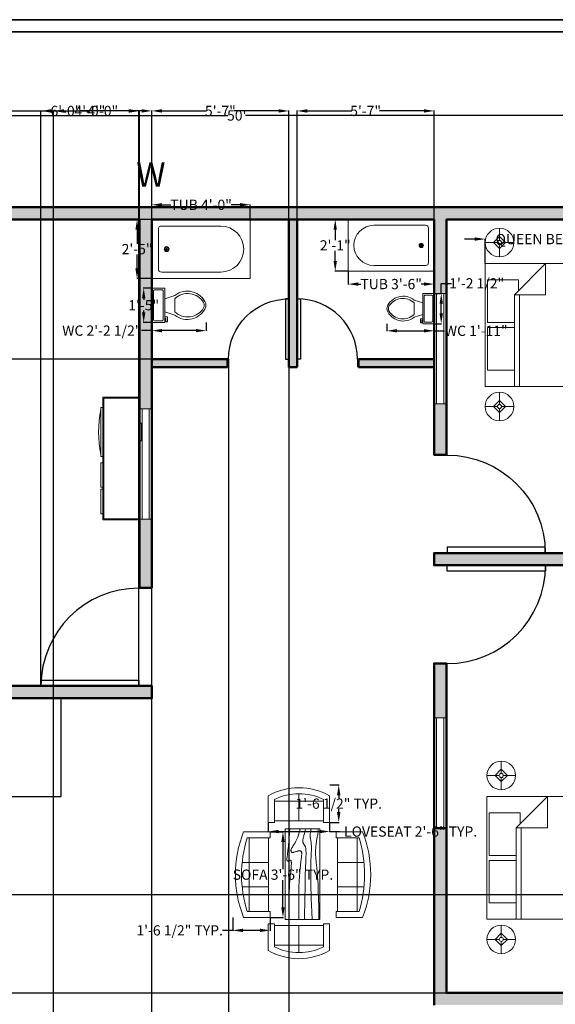
# Model space of a CAD drawing. Units: inches. Extents: x -60 to 743, y -483 to 510.
# Tile 6 of 7: x 209 to 470, y 29 to 510. Entities that reach past the tile are written whole.
import ezdxf

# ---------------------------------------------------------------- set-up
doc = ezdxf.new("R2010")
doc.units = ezdxf.units.IN
doc.header["$MEASUREMENT"] = 0
for name, color, linetype, lineweight in [('A-ANNO-DIMS', 2, 'Continuous', 18), ('A-ANNO-SYMB', 7, 'Continuous', 18), ('A-ANNO-TTLB', 7, 'Continuous', 35), ('A-DOOR', 150, 'Continuous', 25), ('A-FLOR-FIXT', 40, 'Continuous', 18), ('A-WALL-PATT', 30, 'Continuous', 13), ('FURNITURE', 40, 'Continuous', 18), ('STAIRS', 202, 'Continuous', 25), ('WALL BOUNDRY', 10, 'Continuous', 50), ('WINDOW', 200, 'Continuous', 18)]:
    doc.layers.add(name, color=color, linetype=linetype, lineweight=lineweight)
doc.styles.get("Standard").update_dxf_attribs({"font": 'arial.ttf'})
doc.dimstyles.get("Standard").update_dxf_attribs({"dimtxt": 5, "dimasz": 5, "dimexe": 0.18, "dimexo": 0.0625, "dimgap": 0.09, "dimtad": 0, "dimtih": 1, "dimtoh": 1, "dimdec": 1, "dimzin": 0, "dimdsep": 46, "dimlunit": 4, "dimtxsty": 'Standard', "dimcen": 0.09, "dimadec": 0, "dimazin": 0, "dimtfac": 1, "dimtdec": 1, "dimtofl": 0, "dimtmove": 0, "dimatfit": 3, "dimfxl": 1, "dimtolj": 1, "dimtzin": 0, "dimarcsym": 0})

# ---------------------------------------------------------------- blocks, each defined once
blk = doc.blocks.new('*U5')
for p, q in [((0, 0), (0, -100)), ((750, 0), (750, -100))]:
    blk.add_line(p, q)
blk.add_lwpolyline([(0, 0), (0, 750), (43.75, 750), (43.75, 0)], close=True)
blk.add_arc((0, 0), 750, 0, 90)
blk = doc.blocks.new('Sofa - Roundback 7 ft.')
for p, q in [((-12.00002, -32.4421), (-12.00003, -6.5971)), ((11.99997, -32.4421), (11.99998, -6.5971)), ((-36.000027, -34), (-36.000027, -11.4696)), ((-35.999844, -13.3819), (35.9998, -13.3819)), ((35.99998, -34), (35.99998, -11.4696)), ((-36.000027, -32.4421), (35.99998, -32.4421))]:
    blk.add_line(p, q)
for points in [[(-36.000027, -34), (-42.000027, -34), (-42.000027, -8)], [(41.99998, -8), (41.99998, -34), (35.99998, -34)]]:
    blk.add_lwpolyline(points)
for centre, radius, start, end in [((0, -114.25), 114.25, 68.43141, 111.5686), ((-0.00001, -127.1968), 121.1968, 72.72033, 107.2797)]:
    blk.add_arc(centre, radius, start, end)
blk = doc.blocks.new('Sofa - Roundback Loveseat 5 ft.')
for p, q in [((0, -32.44198), (0, -5.99998)), ((-24, -33.99998), (-24, -11.46958)), ((-23.9998, -13.38178), (23.99986, -13.38178)), ((24.00004, -33.99998), (24.00004, -11.46958)), ((-24, -32.44198), (24.00004, -32.44198))]:
    blk.add_line(p, q)
for points in [[(-24, -33.99998), (-30, -33.99998), (-30, -7.99998)], [(30.00004, -7.99998), (30.00004, -33.99998), (24.00004, -33.99998)]]:
    blk.add_lwpolyline(points)
for centre, radius, start, end in [((0, -60.24998), 60.24998, 60.13715, 119.8628), ((0, -61.38438), 55.38444, 64.32083, 115.6792)]:
    blk.add_arc(centre, radius, start, end)
blk = doc.blocks.new('Lamp - Table')
for p, q in [((0, 7), (0, 1)), ((-1, 0), (-7, 0)), ((0, 3), (-3, 0)), ((-3, 0), (0, -3)), ((3, 0), (0, 3)), ((0, -3), (3, 0)), ((1, 0), (7, 0)), ((0, -1), (0, -7))]:
    blk.add_line(p, q)
for radius in [7, 1]:
    blk.add_circle((0, 0), radius)
blk = doc.blocks.new('Bed - Queen')
for p, q in [((0, -80.00003), (0, 0)), ((0, 0), (59.99999, 0)), ((59.99999, 0), (59.99999, -80.00003)), ((7.99999, -1.2), (28.79998, -1.2)), ((7.99999, -14.4), (7.99999, -1.2)), ((28.79998, -1.2), (28.79998, -14.4)), ((31.19999, -1.2), (51.99999, -1.2)), ((31.19999, -14.4), (31.19999, -1.2)), ((51.99999, -1.2), (51.99999, -16.4)), ((0, -14.4), (44.8, -14.4)), ((59.99999, -29.6), (44.8, -14.4)), ((44.8, -14.4), (44.8, -29.6)), ((44.8, -16.8), (0, -16.8)), ((51.99999, -16.4), (46.79936, -16.4)), ((44.8, -29.6), (59.99999, -29.6)), ((59.99999, -80.00003), (0, -80.00003))]:
    blk.add_line(p, q)
blk = doc.blocks.new('Bath Tub - 26 x 60 in.')
for p, q in [((9, -17), (9, -19)), ((8, -18), (10, -18))]:
    blk.add_line(p, q)
blk.add_lwpolyline([(0, -36), (0, 0), (60, 0), (60, -36)], close=True)
for points in [[(6, -4), (42, -4)], [(4, -30), (4, -6)], [(42, -32), (6, -32)]]:
    blk.add_lwpolyline(points)
for radius in [1.5, 1]:
    blk.add_circle((9, -18), radius)
for centre, radius, start, end in [((5.75, -5.75), 1.77, 81.8699, 188.1301), ((42, -18), 14, 270, 90), ((5.75, -30.25), 1.77, 171.8699, 278.1301)]:
    blk.add_arc(centre, radius, start, end)
blk = doc.blocks.new('Toilet - top')
for p, q in [((9.5, -6), (9.5, -2)), ((-10, -8.5), (-8, -8.5)), ((-10, -9.5), (-10, -8.5)), ((-7, -9.5), (-10, -9.5)), ((-8, -8.5), (-8, -8)), ((-7, -8), (-7, -9.5)), ((-4, -8), (-6, -14)), ((4, -8), (6, -14)), ((4, -14), (-4, -14))]:
    blk.add_line(p, q)
blk.add_lwpolyline([(10.5, -8), (10.5, 0), (-10.5, 0), (-10.5, -8)], close=True)
for points in [[(-9.5, -2), (-9.5, -6)], [(8.5, -1), (-8.5, -1)], [(-8.5, -7), (8.5, -7)]]:
    blk.add_lwpolyline(points)
for centre, radius, start, end in [((-8.62, -1.88), 0.884, 81.8699, 188.1301), ((8.62, -1.88), 0.884, 351.8699, 98.1301), ((-8.62, -6.12), 0.884, 171.8699, 278.1301), ((8.62, -6.12), 0.884, 261.8699, 8.1301), ((3.52, -21.58), 12.17, 141.46911, 247.97143), ((4.2, -21.82), 11.33, 136.36773, 238.94682), ((-3.52, -21.58), 12.17, 292.02843, 38.53071), ((-4.2, -21.82), 11.33, 301.05301, 43.63209), ((0, -27.88), 4, 245.73182, 294.26817), ((0, -29), 4, 254.86053, 285.13947)]:
    blk.add_arc(centre, radius, start, end)
blk = doc.blocks.new('Entertainment Center')
for p, q in [((-4, 0), (-5, -1)), ((4, 0), (-4, 0)), ((5, -1), (4, 0)), ((-17, -19), (-17, -1)), ((-17, -1), (43, -1)), ((-16.5, -18.5), (-16.5, -1.5)), ((-16.5, -1.5), (42.5, -1.5)), ((42.5, -1.5), (42.5, -18.5)), ((43, -1), (43, -19)), ((43, -19), (-17, -19)), ((42.5, -18.5), (-16.5, -18.5)), ((-12, -20), (-12, -19)), ((12, -19), (12, -20)), ((15, -20), (15, -19)), ((27, -19), (27, -20)), ((28, -20), (28, -19)), ((40, -19), (40, -20)), ((12, -20), (-12, -20)), ((27, -20), (15, -20)), ((40, -20), (28, -20))]:
    blk.add_line(p, q)
blk.add_arc((0, 40), 61, 259.6111, 280.3889)
blk = doc.blocks.new('*D22')
at = {"layer": 'A-ANNO-DIMS', "color": 0, "lineweight": -2, "transparency": 16777216}
for p, q in [((13.15, 418.48), (13.15, 463.48)), ((18.15, 463.3), (310.31, 463.3)), ((611.15, 463.3), (318.98, 463.3)), ((616.15, 418.48), (616.15, 463.48))]:
    blk.add_line(p, q, dxfattribs=at)
at = {"layer": 'A-ANNO-DIMS', "color": 0, "transparency": 16777216}
for points in [[(18.15, 464.13), (18.15, 462.46), (13.15, 463.3)], [(611.15, 464.13), (611.15, 462.46), (616.15, 463.3)]]:
    blk.add_solid(points, dxfattribs=at)
at = {"layer": 'Defpoints', "color": 0, "transparency": 16777216}
for p in [(616.15, 463.3), (13.15, 418.42), (616.15, 418.42)]:
    blk.add_point(p, dxfattribs=at)
at = {"layer": 'A-ANNO-DIMS', "color": 0, "transparency": 16777216, "insert": (314.65, 463.3), "char_height": 5, "attachment_point": 5}
blk.add_mtext("\\A1;50'", dxfattribs=at)
blk = doc.blocks.new('*D40')
at = {"layer": 'A-ANNO-DIMS', "color": 0, "lineweight": -2, "transparency": 16777216}
for p, q in [((273.15, 412.48), (273.15, 419.82)), ((278.15, 419.64), (282.46, 419.64)), ((316.28, 419.64), (311.97, 419.64)), ((321.28, 412.48), (321.28, 419.82))]:
    blk.add_line(p, q, dxfattribs=at)
at = {"layer": 'A-ANNO-DIMS', "color": 0, "transparency": 16777216}
for points in [[(278.15, 420.48), (278.15, 418.81), (273.15, 419.64)], [(316.28, 420.48), (316.28, 418.81), (321.28, 419.64)]]:
    blk.add_solid(points, dxfattribs=at)
at = {"layer": 'Defpoints', "color": 0, "transparency": 16777216}
for p in [(321.28, 419.64), (273.15, 412.42), (321.28, 412.42)]:
    blk.add_point(p, dxfattribs=at)
at = {"layer": 'A-ANNO-DIMS', "color": 0, "transparency": 16777216, "insert": (297.21, 419.64), "char_height": 5, "attachment_point": 5}
blk.add_mtext('\\A1;TUB 4\'-0"', dxfattribs=at)
blk = doc.blocks.new('*D41')
at = {"layer": 'A-ANNO-DIMS', "color": 0, "lineweight": -2, "transparency": 16777216}
for p, q in [((273.08, 412.42), (265.75, 412.42)), ((265.93, 407.42), (265.93, 400.62)), ((265.93, 388.54), (265.93, 395.34)), ((273.08, 383.54), (265.75, 383.54))]:
    blk.add_line(p, q, dxfattribs=at)
at = {"layer": 'A-ANNO-DIMS', "color": 0, "transparency": 16777216}
for points in [[(265.09, 407.42), (266.76, 407.42), (265.93, 412.42)], [(265.09, 388.54), (266.76, 388.54), (265.93, 383.54)]]:
    blk.add_solid(points, dxfattribs=at)
at = {"layer": 'Defpoints', "color": 0, "transparency": 16777216}
for p in [(265.93, 412.42), (273.15, 412.42), (273.15, 383.54)]:
    blk.add_point(p, dxfattribs=at)
at = {"layer": 'A-ANNO-DIMS', "color": 0, "transparency": 16777216, "insert": (265.93, 397.98), "char_height": 5, "attachment_point": 5}
blk.add_mtext('\\A1;2\'-5"', dxfattribs=at)
blk = doc.blocks.new('*D42')
at = {"layer": 'A-ANNO-DIMS', "color": 0, "lineweight": -2, "transparency": 16777216}
for p, q in [((369.11, 387.13), (369.11, 380.71)), ((411.15, 387.13), (411.15, 380.71)), ((374.11, 380.89), (375.37, 380.89)), ((406.15, 380.89), (404.88, 380.89))]:
    blk.add_line(p, q, dxfattribs=at)
at = {"layer": 'A-ANNO-DIMS', "color": 0, "transparency": 16777216}
for points in [[(374.11, 381.72), (374.11, 380.06), (369.11, 380.89)], [(406.15, 381.72), (406.15, 380.06), (411.15, 380.89)]]:
    blk.add_solid(points, dxfattribs=at)
at = {"layer": 'Defpoints', "color": 0, "transparency": 16777216}
for p in [(369.11, 387.2), (411.15, 387.2), (369.11, 380.89)]:
    blk.add_point(p, dxfattribs=at)
at = {"layer": 'A-ANNO-DIMS', "color": 0, "transparency": 16777216, "insert": (390.13, 380.89), "char_height": 5, "attachment_point": 5}
blk.add_mtext('\\A1;TUB 3\'-6"', dxfattribs=at)
blk = doc.blocks.new('*D43')
at = {"layer": 'A-ANNO-DIMS', "color": 0, "lineweight": -2, "transparency": 16777216}
for p, q in [((369.04, 412.42), (362.62, 412.42)), ((362.8, 407.42), (362.8, 402.41)), ((362.8, 392.2), (362.8, 397.21)), ((369.04, 387.2), (362.62, 387.2))]:
    blk.add_line(p, q, dxfattribs=at)
at = {"layer": 'A-ANNO-DIMS', "color": 0, "transparency": 16777216}
for points in [[(361.97, 407.42), (363.63, 407.42), (362.8, 412.42)], [(361.97, 392.2), (363.63, 392.2), (362.8, 387.2)]]:
    blk.add_solid(points, dxfattribs=at)
at = {"layer": 'Defpoints', "color": 0, "transparency": 16777216}
for p in [(362.8, 412.42), (369.11, 412.42), (369.11, 387.2)]:
    blk.add_point(p, dxfattribs=at)
at = {"layer": 'A-ANNO-DIMS', "color": 0, "transparency": 16777216, "insert": (362.8, 399.81), "char_height": 5, "attachment_point": 5}
blk.add_mtext('\\A1;2\'-1"', dxfattribs=at)
blk = doc.blocks.new('*D46')
at = {"layer": 'A-ANNO-DIMS', "color": 0, "lineweight": -2, "transparency": 16777216}
for p, q in [((273.15, 362.04), (273.15, 357.95)), ((299.66, 362.04), (299.66, 357.95)), ((273.15, 358.13), (268.15, 358.13)), ((294.66, 358.13), (278.15, 358.13))]:
    blk.add_line(p, q, dxfattribs=at)
at = {"layer": 'A-ANNO-DIMS', "color": 0, "transparency": 16777216}
for points in [[(278.15, 358.96), (278.15, 357.3), (273.15, 358.13)], [(294.66, 358.96), (294.66, 357.3), (299.66, 358.13)]]:
    blk.add_solid(points, dxfattribs=at)
at = {"layer": 'Defpoints', "color": 0, "transparency": 16777216}
for p in [(273.15, 362.11), (299.66, 362.11), (273.15, 358.13)]:
    blk.add_point(p, dxfattribs=at)
at = {"layer": 'A-ANNO-DIMS', "color": 0, "transparency": 16777216, "insert": (248.69, 358.13), "char_height": 5, "attachment_point": 5}
blk.add_mtext('\\A1;WC 2\'-2 1/2"', dxfattribs=at)
blk = doc.blocks.new('*D47')
at = {"layer": 'A-ANNO-DIMS', "color": 0, "lineweight": -2, "transparency": 16777216}
for p, q in [((273.08, 378.95), (268.99, 378.95)), ((269.17, 373.95), (269.17, 373.17)), ((269.17, 367.11), (269.17, 367.89)), ((273.08, 362.11), (268.99, 362.11))]:
    blk.add_line(p, q, dxfattribs=at)
at = {"layer": 'A-ANNO-DIMS', "color": 0, "transparency": 16777216}
for points in [[(268.34, 373.95), (270, 373.95), (269.17, 378.95)], [(268.34, 367.11), (270, 367.11), (269.17, 362.11)]]:
    blk.add_solid(points, dxfattribs=at)
at = {"layer": 'Defpoints', "color": 0, "transparency": 16777216}
for p in [(269.17, 378.95), (273.15, 378.95), (273.15, 362.11)]:
    blk.add_point(p, dxfattribs=at)
at = {"layer": 'A-ANNO-DIMS', "color": 0, "transparency": 16777216, "insert": (269.17, 370.53), "char_height": 5, "attachment_point": 5}
blk.add_mtext('\\A1;1\'-5"', dxfattribs=at)
blk = doc.blocks.new('*D48')
at = {"layer": 'A-ANNO-DIMS', "color": 0, "lineweight": -2, "transparency": 16777216}
for p, q in [((387.99, 361.46), (387.99, 357.87)), ((411.15, 361.46), (411.15, 357.87)), ((392.99, 358.05), (406.15, 358.05)), ((411.15, 358.05), (416.15, 358.05))]:
    blk.add_line(p, q, dxfattribs=at)
at = {"layer": 'A-ANNO-DIMS', "color": 0, "transparency": 16777216}
for points in [[(392.99, 358.88), (392.99, 357.22), (387.99, 358.05)], [(406.15, 358.88), (406.15, 357.22), (411.15, 358.05)]]:
    blk.add_solid(points, dxfattribs=at)
at = {"layer": 'Defpoints', "color": 0, "transparency": 16777216}
for p in [(387.99, 361.52), (411.15, 361.52), (411.15, 358.05)]:
    blk.add_point(p, dxfattribs=at)
at = {"layer": 'A-ANNO-DIMS', "color": 0, "transparency": 16777216, "insert": (431.72, 358.05), "char_height": 5, "attachment_point": 5}
blk.add_mtext('\\A1;WC 1\'-11"', dxfattribs=at)
blk = doc.blocks.new('*D49')
at = {"layer": 'A-ANNO-DIMS', "color": 0, "lineweight": -2, "transparency": 16777216}
for p, q in [((414.62, 376.24), (414.62, 381.24)), ((414.62, 381.24), (419.62, 381.24)), ((411.21, 376.24), (414.8, 376.24)), ((414.62, 366.52), (414.62, 371.24)), ((411.21, 361.52), (414.8, 361.52))]:
    blk.add_line(p, q, dxfattribs=at)
at = {"layer": 'A-ANNO-DIMS', "color": 0, "transparency": 16777216}
for points in [[(413.79, 371.24), (415.45, 371.24), (414.62, 376.24)], [(413.79, 366.52), (415.45, 366.52), (414.62, 361.52)]]:
    blk.add_solid(points, dxfattribs=at)
at = {"layer": 'Defpoints', "color": 0, "transparency": 16777216}
for p in [(411.15, 376.24), (414.62, 376.24), (411.15, 361.52)]:
    blk.add_point(p, dxfattribs=at)
at = {"layer": 'A-ANNO-DIMS', "color": 0, "transparency": 16777216, "insert": (431.95, 381.24), "char_height": 5, "attachment_point": 5}
blk.add_mtext('\\A1;1\'-2 1/2"', dxfattribs=at)
blk = doc.blocks.new('*D50')
at = {"layer": 'A-ANNO-DIMS', "color": 0, "lineweight": -2, "transparency": 16777216}
for p, q in [((431.03, 402.88), (426.03, 402.88)), ((436.03, 390.95), (436.03, 403.06)), ((516.03, 390.95), (516.03, 403.06)), ((521.03, 402.88), (526.03, 402.88))]:
    blk.add_line(p, q, dxfattribs=at)
at = {"layer": 'A-ANNO-DIMS', "color": 0, "transparency": 16777216}
for points in [[(431.03, 403.72), (431.03, 402.05), (436.03, 402.88)], [(521.03, 403.72), (521.03, 402.05), (516.03, 402.88)]]:
    blk.add_solid(points, dxfattribs=at)
at = {"layer": 'Defpoints', "color": 0, "transparency": 16777216}
for p in [(436.03, 402.88), (436.03, 390.88), (516.03, 390.88)]:
    blk.add_point(p, dxfattribs=at)
at = {"layer": 'A-ANNO-DIMS', "color": 0, "transparency": 16777216, "insert": (476.03, 402.88), "char_height": 5, "attachment_point": 5}
blk.add_mtext('\\A1;QUEEN BED 6\'-8" TYP.', dxfattribs=at)
blk = doc.blocks.new('*D54')
at = {"layer": 'A-ANNO-DIMS', "color": 0, "lineweight": -2, "transparency": 16777216}
for p, q in [((331.03, 113.14), (337.43, 113.14)), ((337.25, 108.14), (337.25, 94.87)), ((337.25, 76.24), (337.25, 89.51)), ((331.03, 71.24), (337.43, 71.24))]:
    blk.add_line(p, q, dxfattribs=at)
at = {"layer": 'A-ANNO-DIMS', "color": 0, "transparency": 16777216}
for points in [[(336.42, 108.14), (338.09, 108.14), (337.25, 113.14)], [(336.42, 76.24), (338.09, 76.24), (337.25, 71.24)]]:
    blk.add_solid(points, dxfattribs=at)
at = {"layer": 'Defpoints', "color": 0, "transparency": 16777216}
for p in [(330.97, 113.14), (330.97, 71.24), (337.25, 71.24)]:
    blk.add_point(p, dxfattribs=at)
at = {"layer": 'A-ANNO-DIMS', "color": 0, "transparency": 16777216, "insert": (337.25, 92.19), "char_height": 5, "attachment_point": 5}
blk.add_mtext('\\A1;SOFA 3\'-6" TYP.', dxfattribs=at)
blk = doc.blocks.new('*D55')
at = {"layer": 'A-ANNO-DIMS', "color": 0, "lineweight": -2, "transparency": 16777216}
for p, q in [((312.68, 71.18), (312.68, 64.77)), ((330.97, 71.18), (330.97, 64.77)), ((312.68, 64.95), (307.68, 64.95)), ((325.97, 64.95), (317.68, 64.95))]:
    blk.add_line(p, q, dxfattribs=at)
at = {"layer": 'A-ANNO-DIMS', "color": 0, "transparency": 16777216}
for points in [[(317.68, 65.79), (317.68, 64.12), (312.68, 64.95)], [(325.97, 65.79), (325.97, 64.12), (330.97, 64.95)]]:
    blk.add_solid(points, dxfattribs=at)
at = {"layer": 'Defpoints', "color": 0, "transparency": 16777216}
for p in [(312.68, 71.24), (330.97, 71.24), (312.68, 64.95)]:
    blk.add_point(p, dxfattribs=at)
at = {"layer": 'A-ANNO-DIMS', "color": 0, "transparency": 16777216, "insert": (286.76, 64.95), "char_height": 5, "attachment_point": 5}
blk.add_mtext('\\A1;1\'-6 1/2" TYP.', dxfattribs=at)
blk = doc.blocks.new('*D56')
at = {"layer": 'A-ANNO-DIMS', "color": 0, "lineweight": -2, "transparency": 16777216}
for p, q in [((330.09, 117.69), (330.09, 113.08)), ((360.02, 117.69), (360.02, 113.08)), ((335.09, 113.26), (355.02, 113.26)), ((360.02, 113.26), (365.02, 113.26))]:
    blk.add_line(p, q, dxfattribs=at)
at = {"layer": 'A-ANNO-DIMS', "color": 0, "transparency": 16777216}
for points in [[(335.09, 114.09), (335.09, 112.43), (330.09, 113.26)], [(355.02, 114.09), (355.02, 112.43), (360.02, 113.26)]]:
    blk.add_solid(points, dxfattribs=at)
at = {"layer": 'Defpoints', "color": 0, "transparency": 16777216}
for p in [(330.09, 117.75), (360.02, 117.75), (360.02, 113.26)]:
    blk.add_point(p, dxfattribs=at)
at = {"layer": 'A-ANNO-DIMS', "color": 0, "transparency": 16777216, "insert": (399.65, 113.26), "char_height": 5, "attachment_point": 5}
blk.add_mtext('\\A1;LOVESEAT 2\'-6" TYP.', dxfattribs=at)
blk = doc.blocks.new('*D57')
at = {"layer": 'A-ANNO-DIMS', "color": 0, "lineweight": -2, "transparency": 16777216}
for p, q in [((360.08, 136.04), (364.69, 136.04)), ((364.51, 131.04), (364.51, 129.57)), ((364.51, 122.75), (364.51, 124.22)), ((360.08, 117.75), (364.69, 117.75))]:
    blk.add_line(p, q, dxfattribs=at)
at = {"layer": 'A-ANNO-DIMS', "color": 0, "transparency": 16777216}
for points in [[(363.67, 131.04), (365.34, 131.04), (364.51, 136.04)], [(363.67, 122.75), (365.34, 122.75), (364.51, 117.75)]]:
    blk.add_solid(points, dxfattribs=at)
at = {"layer": 'Defpoints', "color": 0, "transparency": 16777216}
for p in [(360.02, 136.04), (364.51, 136.04), (360.02, 117.75)]:
    blk.add_point(p, dxfattribs=at)
at = {"layer": 'A-ANNO-DIMS', "color": 0, "transparency": 16777216, "insert": (364.51, 126.9), "char_height": 5, "attachment_point": 5}
blk.add_mtext('\\A1;1\'-6 1/2" TYP.', dxfattribs=at)
blk = doc.blocks.new('*D66')
at = {"layer": 'A-ANNO-DIMS', "color": 0, "lineweight": -2, "transparency": 16777216}
for p, q in [((273.15, 412.48), (273.15, 465.7)), ((278.15, 465.52), (299.91, 465.52)), ((335.15, 465.52), (313.38, 465.52)), ((340.15, 412.48), (340.15, 465.7))]:
    blk.add_line(p, q, dxfattribs=at)
at = {"layer": 'A-ANNO-DIMS', "color": 0, "transparency": 16777216}
for points in [[(278.15, 466.36), (278.15, 464.69), (273.15, 465.52)], [(335.15, 466.36), (335.15, 464.69), (340.15, 465.52)]]:
    blk.add_solid(points, dxfattribs=at)
at = {"layer": 'Defpoints', "color": 0, "transparency": 16777216}
for p in [(340.15, 465.52), (273.15, 412.42), (340.15, 412.42)]:
    blk.add_point(p, dxfattribs=at)
at = {"layer": 'A-ANNO-DIMS', "color": 0, "transparency": 16777216, "insert": (306.65, 465.52), "char_height": 5, "attachment_point": 5}
blk.add_mtext('\\A1;5\'-7"', dxfattribs=at)
blk = doc.blocks.new('*D67')
at = {"layer": 'A-ANNO-DIMS', "color": 0, "lineweight": -2, "transparency": 16777216}
for p, q in [((344.15, 412.48), (344.15, 465.7)), ((349.15, 465.52), (370.91, 465.52)), ((406.15, 465.52), (384.38, 465.52)), ((411.15, 412.48), (411.15, 465.7))]:
    blk.add_line(p, q, dxfattribs=at)
at = {"layer": 'A-ANNO-DIMS', "color": 0, "transparency": 16777216}
for points in [[(349.15, 466.36), (349.15, 464.69), (344.15, 465.52)], [(406.15, 466.36), (406.15, 464.69), (411.15, 465.52)]]:
    blk.add_solid(points, dxfattribs=at)
at = {"layer": 'Defpoints', "color": 0, "transparency": 16777216}
for p in [(411.15, 465.52), (344.15, 412.42), (411.15, 412.42)]:
    blk.add_point(p, dxfattribs=at)
at = {"layer": 'A-ANNO-DIMS', "color": 0, "transparency": 16777216, "insert": (377.65, 465.52), "char_height": 5, "attachment_point": 5}
blk.add_mtext('\\A1;5\'-7"', dxfattribs=at)
blk = doc.blocks.new('*D68')
at = {"layer": 'A-ANNO-DIMS', "color": 0, "lineweight": -2, "transparency": 16777216}
for p, q in [((273.08, 412.42), (-36.93, 412.42)), ((-36.75, 407.42), (-36.75, 380.97)), ((-36.75, 349.23), (-36.75, 375.68)), ((273.08, 344.23), (-36.93, 344.23))]:
    blk.add_line(p, q, dxfattribs=at)
at = {"layer": 'A-ANNO-DIMS', "color": 0, "transparency": 16777216}
for points in [[(-37.58, 407.42), (-35.91, 407.42), (-36.75, 412.42)], [(-37.58, 349.23), (-35.91, 349.23), (-36.75, 344.23)]]:
    blk.add_solid(points, dxfattribs=at)
at = {"layer": 'Defpoints', "color": 0, "transparency": 16777216}
for p in [(273.15, 412.42), (-36.75, 344.23), (273.15, 344.23)]:
    blk.add_point(p, dxfattribs=at)
at = {"layer": 'A-ANNO-DIMS', "color": 0, "transparency": 16777216, "insert": (-36.75, 378.32), "char_height": 5, "attachment_point": 5}
blk.add_mtext('\\A1;5\'-8"', dxfattribs=at)
blk = doc.blocks.new('*D69')
at = {"layer": 'A-ANNO-DIMS', "color": 0, "lineweight": -2, "transparency": 16777216}
for p, q in [((310.62, 340.16), (310.62, -473.51)), ((340.15, 340.16), (340.15, -473.51)), ((305.62, -473.33), (300.62, -473.33)), ((345.15, -473.33), (350.15, -473.33))]:
    blk.add_line(p, q, dxfattribs=at)
at = {"layer": 'A-ANNO-DIMS', "color": 0, "transparency": 16777216}
for points in [[(305.62, -472.5), (305.62, -474.17), (310.62, -473.33)], [(345.15, -472.5), (345.15, -474.17), (340.15, -473.33)]]:
    blk.add_solid(points, dxfattribs=at)
at = {"layer": 'Defpoints', "color": 0, "transparency": 16777216}
for p in [(310.62, 340.23), (340.15, 340.23), (340.15, -473.33)]:
    blk.add_point(p, dxfattribs=at)
at = {"layer": 'A-ANNO-DIMS', "color": 0, "transparency": 16777216, "insert": (325.38, -473.33), "char_height": 5, "attachment_point": 5}
blk.add_mtext('\\A1;2\'-5 1/2"', dxfattribs=at)
blk = doc.blocks.new('*D74')
at = {"layer": 'A-ANNO-DIMS', "color": 0, "lineweight": -2, "transparency": 16777216}
for p, q in [((187.21, 82.42), (679.73, 82.42)), ((679.55, 77.42), (679.55, 61.06)), ((679.55, 39.42), (679.55, 55.78)), ((187.21, 34.42), (679.73, 34.42))]:
    blk.add_line(p, q, dxfattribs=at)
at = {"layer": 'A-ANNO-DIMS', "color": 0, "transparency": 16777216}
for points in [[(678.72, 77.42), (680.39, 77.42), (679.55, 82.42)], [(678.72, 39.42), (680.39, 39.42), (679.55, 34.42)]]:
    blk.add_solid(points, dxfattribs=at)
at = {"layer": 'Defpoints', "color": 0, "transparency": 16777216}
for p in [(187.15, 82.42), (679.55, 82.42), (187.15, 34.42)]:
    blk.add_point(p, dxfattribs=at)
at = {"layer": 'A-ANNO-DIMS', "color": 0, "transparency": 16777216, "insert": (679.55, 58.42), "char_height": 5, "attachment_point": 5}
blk.add_mtext('\\A1;4\'-0"', dxfattribs=at)
blk = doc.blocks.new('*D75')
at = {"layer": 'A-ANNO-DIMS', "color": 0, "lineweight": -2, "transparency": 16777216}
for p, q in [((218.96, 184.48), (218.96, 465.7)), ((223.96, 465.52), (236.03, 465.52)), ((261.77, 465.52), (249.7, 465.52)), ((266.77, 184.48), (266.77, 465.7))]:
    blk.add_line(p, q, dxfattribs=at)
at = {"layer": 'A-ANNO-DIMS', "color": 0, "transparency": 16777216}
for points in [[(223.96, 466.36), (223.96, 464.69), (218.96, 465.52)], [(261.77, 466.36), (261.77, 464.69), (266.77, 465.52)]]:
    blk.add_solid(points, dxfattribs=at)
at = {"layer": 'Defpoints', "color": 0, "transparency": 16777216}
for p in [(266.77, 465.52), (218.96, 184.42), (266.77, 184.42)]:
    blk.add_point(p, dxfattribs=at)
at = {"layer": 'A-ANNO-DIMS', "color": 0, "transparency": 16777216, "insert": (242.87, 465.52), "char_height": 5, "attachment_point": 5}
blk.add_mtext('\\A1;4\'-0"', dxfattribs=at)
blk = doc.blocks.new('*D78')
at = {"layer": 'A-ANNO-DIMS', "color": 0, "lineweight": -2, "transparency": 16777216}
for p, q in [((225.15, -143.52), (225.15, 465.7)), ((230.15, 465.52), (242.31, 465.52)), ((268.15, 465.52), (255.98, 465.52)), ((273.15, -143.91), (273.15, 465.7))]:
    blk.add_line(p, q, dxfattribs=at)
at = {"layer": 'A-ANNO-DIMS', "color": 0, "transparency": 16777216}
for points in [[(230.15, 466.36), (230.15, 464.69), (225.15, 465.52)], [(268.15, 466.36), (268.15, 464.69), (273.15, 465.52)]]:
    blk.add_solid(points, dxfattribs=at)
at = {"layer": 'Defpoints', "color": 0, "transparency": 16777216}
for p in [(273.15, 465.52), (225.15, -143.58), (273.15, -143.98)]:
    blk.add_point(p, dxfattribs=at)
at = {"layer": 'A-ANNO-DIMS', "color": 0, "transparency": 16777216, "insert": (249.15, 465.52), "char_height": 5, "attachment_point": 5}
blk.add_mtext('\\A1;4\'-0"', dxfattribs=at)
blk = doc.blocks.new('*D81')
at = {"layer": 'A-ANNO-DIMS', "color": 0, "lineweight": -2, "transparency": 16777216}
for p, q in [((195.14, 348.96), (195.14, 465.7)), ((200.14, 465.52), (224.39, 465.52)), ((262.15, 465.52), (237.89, 465.52)), ((267.15, 412.48), (267.15, 465.7))]:
    blk.add_line(p, q, dxfattribs=at)
at = {"layer": 'A-ANNO-DIMS', "color": 0, "transparency": 16777216}
for points in [[(200.14, 466.36), (200.14, 464.69), (195.14, 465.52)], [(262.15, 466.36), (262.15, 464.69), (267.15, 465.52)]]:
    blk.add_solid(points, dxfattribs=at)
at = {"layer": 'Defpoints', "color": 0, "transparency": 16777216}
for p in [(267.15, 465.52), (267.15, 412.42), (195.14, 348.9)]:
    blk.add_point(p, dxfattribs=at)
at = {"layer": 'A-ANNO-DIMS', "color": 0, "transparency": 16777216, "insert": (231.14, 465.52), "char_height": 5, "attachment_point": 5}
blk.add_mtext('\\A1;6\'-0"', dxfattribs=at)

msp = doc.modelspace()

# ---------------------------------------------------------------- hatches: boundary and pattern name
at = {"layer": 'A-WALL-PATT'}
h = msp.add_hatch(color=256, dxfattribs=at)
h.dxf.hatch_style = 1
h.paths.add_polyline_path([(412.35, 168.77), (415.89, 168.77), (415.89, 114.92), (412.35, 114.92)], flags=16)
h.paths.add_polyline_path([(87.81, -138.81), (87.81, -142.35), (48.31, -142.32), (48.31, -138.78)], flags=16)
h.paths.add_polyline_path([(459.53, -138.78), (513.39, -138.78), (513.39, -142.32), (459.53, -142.32)], flags=16)
h.paths.add_polyline_path([(164.84, -257.78), (218.7, -257.78), (218.7, -261.32), (164.84, -261.32)], flags=16)
h.paths.add_polyline_path([(417.15, 114.92), (415.89, 114.92), (415.89, 168.77), (417.15, 168.77), (417.15, 195.42), (411.15, 195.42), (411.15, 168.77), (412.35, 168.77), (412.35, 114.92), (411.15, 114.92), (411.15, 28.42), (610.15, 28.42), (610.15, -43.58), (508.15, -43.58), (508.15, -49.58), (610.15, -49.58), (610.15, -137.58), (513.39, -137.58), (513.39, -138.78), (459.53, -138.78), (459.53, -137.58), (359.15, -137.58), (359.15, -143.58), (377.15, -143.58), (377.15, -292.58), (383.15, -292.58), (383.15, -143.58), (459.53, -143.58), (459.53, -142.32), (513.39, -142.32), (513.39, -143.58), (610.15, -143.58), (610.15, -415.58), (610.15, -421.58), (616.15, -421.58), (616.15, 418.42), (13.15, 418.42), (13.15, -421.58), (19.15, -421.58), (430.15, -421.58), (430.15, -415.58), (19.15, -415.58), (19.15, -143.58), (48.31, -143.58), (48.31, -142.32), (87.81, -142.35), (87.81, -143.58), (117.15, -143.58), (117.15, -262.58), (164.84, -262.58), (164.84, -261.32), (218.7, -261.32), (218.7, -262.58), (273.15, -262.58), (273.15, -292.58), (279.15, -292.58), (279.15, -143.58), (297.15, -143.58), (297.15, -137.58), (273.15, -137.58), (273.15, -256.58), (218.7, -256.58), (218.7, -257.78), (164.84, -257.78), (164.84, -256.58), (123.15, -256.58), (123.15, -143.58), (225.15, -143.58), (225.15, -137.58), (87.81, -137.58), (87.81, -138.81), (48.31, -138.78), (48.31, -137.58), (19.15, -137.58), (19.15, 28.42), (187.15, 28.42), (187.15, 34.42), (19.15, 34.42), (19.15, 178.42), (273.15, 178.42), (273.15, 184.42), (19.15, 184.42), (19.15, 345.58), (195.14, 345.58), (195.14, 348.9), (19.15, 348.9), (19.15, 412.42), (267.15, 412.42), (267.15, 319.83), (273.15, 319.83), (273.15, 412.42), (411.15, 412.42), (411.15, 376.24), (417.15, 376.24), (417.15, 412.42), (610.15, 412.42), (610.15, 249.42), (411.15, 249.42), (411.15, 243.42), (610.15, 243.42), (610.15, 34.42), (417.15, 34.42)])
h = msp.add_hatch(color=256, dxfattribs=at)
h.dxf.hatch_style = 1
h.paths.add_polyline_path([(344.15, 412.42), (340.15, 412.42), (340.15, 340.23), (344.15, 340.23)])
h.paths.add_polyline_path([(310.15, 344.23), (273.15, 344.23), (273.15, 340.23), (310.15, 340.23)])
h.paths.add_polyline_path([(411.15, 344.23), (374.15, 344.23), (374.15, 340.23), (411.15, 340.23)])
h = msp.add_hatch(color=256, dxfattribs=at)
h.dxf.hatch_style = 1
h.paths.add_polyline_path([(273.15, 265.98), (267.15, 265.98), (267.15, 232.42), (273.15, 232.42)])
h.paths.add_polyline_path([(417.15, 322.39), (411.15, 322.39), (411.15, 297.42), (417.15, 297.42)])
h.paths.add_polyline_path([(417.15, 195.42), (411.15, 195.42), (411.15, 168.77), (417.15, 168.77)])
h.paths.add_polyline_path([(459.53, -137.58), (359.15, -137.58), (359.15, -143.58), (377.15, -143.58), (377.15, -292.58), (383.15, -292.58), (383.15, -143.58), (459.53, -143.58)])
h.paths.add_polyline_path([(279.15, -143.58), (297.15, -143.58), (297.15, -137.58), (273.15, -137.58), (273.15, -256.58), (218.7, -256.58), (218.7, -262.58), (273.15, -262.58), (273.15, -292.58), (279.15, -292.58)])
h.paths.add_polyline_path([(123.15, -143.58), (225.15, -143.58), (225.15, -137.58), (87.81, -137.58), (87.81, -143.58), (117.15, -143.58), (117.15, -262.58), (164.84, -262.58), (164.84, -256.58), (123.15, -256.58)])

# ---------------------------------------------------------------- linework, layer by layer
at = {"layer": 'A-ANNO-TTLB'}
for points in [[(742.84, -483.31), (-60.19, -483.31), (-60.19, 510.12), (742.84, 510.12)], [(736.84, -477.31), (-54.19, -477.31), (-54.19, 504.12), (736.84, 504.12)]]:
    msp.add_lwpolyline(points, close=True, dxfattribs=at)
at = {"layer": 'FURNITURE'}
msp.add_lwpolyline([(355.21, 70.21), (355.21, 114.59), (338.26, 114.59), (338.26, 70.21)], close=True, dxfattribs=at)
for points in [[(340.04, 70.21), (340.05, 73.77), (340.09, 76.88), (340.15, 79.61), (340.22, 81.98), (340.31, 84.05), (340.41, 85.87), (340.52, 87.49), (340.63, 88.94), (340.74, 90.29), (340.85, 91.52), (340.95, 92.65), (341.05, 93.67), (341.14, 94.6), (341.21, 95.42), (341.28, 96.14), (341.32, 96.76), (341.35, 97.29), (341.36, 97.72), (341.35, 98.08), (341.33, 98.37), (341.3, 98.6), (341.25, 98.78), (341.19, 98.92), (341.12, 99.03), (341.05, 99.11), (340.96, 99.17), (340.87, 99.21), (340.77, 99.23), (340.68, 99.24), (340.58, 99.23), (340.48, 99.21), (340.38, 99.18), (340.29, 99.13), (340.21, 99.09), (340.13, 99.04), (340.05, 98.98), (339.97, 98.94), (339.89, 98.89), (339.82, 98.86), (339.74, 98.83), (339.67, 98.82), (339.6, 98.82), (339.53, 98.84), (339.46, 98.87), (339.4, 98.91), (339.34, 98.97), (339.29, 99.04), (339.25, 99.13), (339.22, 99.23), (339.2, 99.34), (339.18, 99.48), (339.18, 99.64), (339.18, 99.83), (339.2, 100.06), (339.22, 100.31), (339.25, 100.61), (339.29, 100.94), (339.34, 101.33), (339.4, 101.77), (339.47, 102.27), (339.54, 102.85), (339.62, 103.5), (339.7, 104.24), (339.79, 105.07), (339.89, 105.99), (339.99, 107.01), (340.09, 108.11), (340.19, 109.29), (340.3, 110.53), (340.41, 111.84), (340.52, 113.19), (340.63, 114.59)], [(345.07, 70.21), (344.98, 75.07), (344.95, 79.04), (344.95, 82.23), (344.99, 84.76), (345.05, 86.77), (345.13, 88.37), (345.22, 89.67), (345.32, 90.82), (345.41, 91.9), (345.49, 92.93), (345.57, 93.91), (345.65, 94.85), (345.73, 95.74), (345.81, 96.58), (345.88, 97.36), (345.96, 98.09), (346.03, 98.77), (346.1, 99.39), (346.17, 99.96), (346.23, 100.48), (346.29, 100.95), (346.34, 101.37), (346.38, 101.75), (346.4, 102.08), (346.41, 102.38), (346.41, 102.64), (346.4, 102.86), (346.37, 103.05), (346.33, 103.21), (346.28, 103.35), (346.22, 103.46), (346.15, 103.56), (346.07, 103.65), (345.98, 103.72), (345.88, 103.78), (345.75, 103.82), (345.61, 103.84), (345.44, 103.85), (345.24, 103.84), (345.02, 103.81), (344.76, 103.77), (344.49, 103.7), (344.19, 103.63), (343.89, 103.55), (343.58, 103.47), (343.29, 103.38), (343.01, 103.3), (342.75, 103.22), (342.53, 103.15), (342.33, 103.09), (342.16, 103.05), (342.01, 103.02), (341.88, 103), (341.77, 103), (341.66, 103.03), (341.57, 103.07), (341.48, 103.14), (341.4, 103.23), (341.32, 103.33), (341.26, 103.46), (341.21, 103.6), (341.18, 103.76), (341.17, 103.93), (341.17, 104.11), (341.2, 104.3), (341.26, 104.51), (341.35, 104.74), (341.48, 105.01), (341.64, 105.32), (341.85, 105.68), (342.1, 106.11), (342.41, 106.6), (342.76, 107.16), (343.16, 107.82), (343.59, 108.59), (344.03, 109.48), (344.48, 110.51), (344.9, 111.69), (345.3, 113.05), (345.66, 114.59)], [(347.73, 70.21), (347.83, 74.04), (347.9, 77.32), (347.96, 80.11), (348, 82.48), (348.02, 84.49), (348.04, 86.19), (348.06, 87.67), (348.08, 88.97), (348.1, 90.16), (348.12, 91.25), (348.15, 92.27), (348.18, 93.22), (348.22, 94.11), (348.25, 94.97), (348.29, 95.8), (348.32, 96.61), (348.36, 97.42), (348.4, 98.23), (348.43, 99.02), (348.46, 99.79), (348.48, 100.54), (348.5, 101.24), (348.52, 101.91), (348.52, 102.53), (348.52, 103.09), (348.5, 103.61), (348.48, 104.07), (348.45, 104.48), (348.41, 104.85), (348.35, 105.18), (348.29, 105.48), (348.23, 105.73), (348.15, 105.96), (348.06, 106.16), (347.97, 106.33), (347.87, 106.49), (347.78, 106.63), (347.68, 106.76), (347.58, 106.89), (347.49, 107.02), (347.4, 107.15), (347.31, 107.29), (347.23, 107.43), (347.16, 107.59), (347.11, 107.76), (347.06, 107.94), (347.02, 108.13), (346.99, 108.35), (346.98, 108.58), (346.98, 108.82), (347, 109.08), (347.02, 109.35), (347.06, 109.63), (347.11, 109.91), (347.17, 110.19), (347.24, 110.47), (347.32, 110.76), (347.41, 111.06), (347.51, 111.4), (347.63, 111.81), (347.77, 112.31), (347.93, 112.92), (348.12, 113.67), (348.32, 114.59)], [(351.58, 70.21), (351.38, 74), (351.21, 77.35), (351.08, 80.32), (350.98, 82.94), (350.91, 85.26), (350.86, 87.32), (350.83, 89.16), (350.81, 90.84), (350.81, 92.39), (350.82, 93.82), (350.83, 95.15), (350.85, 96.38), (350.88, 97.53), (350.91, 98.6), (350.95, 99.61), (350.99, 100.56), (351.02, 101.46), (351.06, 102.31), (351.09, 103.12), (351.12, 103.88), (351.14, 104.59), (351.15, 105.25), (351.15, 105.86), (351.13, 106.42), (351.11, 106.94), (351.07, 107.4), (351.03, 107.82), (350.97, 108.21), (350.92, 108.56), (350.86, 108.89), (350.8, 109.19), (350.74, 109.47), (350.69, 109.74), (350.64, 109.99), (350.6, 110.24), (350.57, 110.49), (350.54, 110.75), (350.53, 111.01), (350.53, 111.29), (350.54, 111.59), (350.57, 111.91), (350.6, 112.24), (350.65, 112.58), (350.7, 112.91), (350.75, 113.23), (350.8, 113.52), (350.85, 113.77), (350.89, 113.97), (350.92, 114.12), (350.94, 114.22), (350.96, 114.29), (350.97, 114.34), (350.98, 114.38), (350.98, 114.43), (350.99, 114.49), (350.99, 114.59)], [(354.83, 70.21), (354.72, 76.13), (354.61, 80.86), (354.5, 84.57), (354.4, 87.4), (354.29, 89.53), (354.19, 91.11), (354.09, 92.31), (353.99, 93.28), (353.9, 94.17), (353.82, 95), (353.74, 95.78), (353.66, 96.51), (353.59, 97.21), (353.52, 97.87), (353.46, 98.51), (353.4, 99.13), (353.35, 99.73), (353.3, 100.32), (353.26, 100.91), (353.23, 101.49), (353.21, 102.08), (353.19, 102.66), (353.19, 103.26), (353.21, 103.86), (353.23, 104.48), (353.27, 105.1), (353.32, 105.72), (353.37, 106.34), (353.44, 106.94), (353.5, 107.52), (353.58, 108.07), (353.65, 108.58), (353.72, 109.06), (353.8, 109.49), (353.87, 109.9), (353.94, 110.29), (354.01, 110.65), (354.08, 111.01), (354.15, 111.36), (354.22, 111.71), (354.28, 112.07), (354.33, 112.44), (354.38, 112.8), (354.4, 113.17), (354.41, 113.54), (354.39, 113.9), (354.33, 114.25), (354.24, 114.59)]]:
    msp.add_lwpolyline(points, dxfattribs=at)
at = {"layer": 'STAIRS'}
for p, q in [((228.81, 130.42), (228.81, 178.42)), ((228.81, 130.42), (228.81, 178.42)), ((187.15, 130.42), (209.13, 130.42)), ((209.13, 130.42), (228.81, 130.42))]:
    msp.add_line(p, q, dxfattribs=at)
at = {"layer": 'WALL BOUNDRY'}
for p, q in [((340.15, 412.42), (340.15, 340.23)), ((344.15, 412.42), (344.15, 340.23)), ((310.15, 344.23), (273.15, 344.23)), ((310.15, 344.23), (310.15, 340.23)), ((374.15, 344.23), (411.15, 344.23)), ((374.15, 344.23), (374.15, 340.23)), ((310.15, 340.23), (273.15, 340.23)), ((340.15, 340.23), (344.15, 340.23)), ((374.15, 340.23), (411.15, 340.23)), ((411.15, 114.92), (417.15, 114.92))]:
    msp.add_line(p, q, dxfattribs=at)
msp.add_lwpolyline([(610.15, -415.58), (610.15, -421.58), (616.15, -421.58), (616.15, 418.42), (13.15, 418.42), (13.15, -421.58), (19.15, -421.58), (430.15, -421.58), (430.15, -415.58), (19.15, -415.58), (19.15, -143.58), (117.15, -143.58), (117.15, -262.58), (273.15, -262.58), (273.15, -292.58), (279.15, -292.58), (377.15, -292.58), (383.15, -292.58), (383.15, -143.58), (610.15, -143.58)], close=True, dxfattribs=at)
for points in [[(187.15, 28.42), (187.15, 34.42), (19.15, 34.42), (19.15, 178.42), (273.15, 178.42), (273.15, 184.42), (19.15, 184.42), (19.15, 345.58), (195.14, 345.58), (195.14, 348.9), (19.15, 348.9), (19.15, 412.42), (267.15, 412.42), (267.15, 232.42), (273.15, 232.42), (273.15, 412.42), (411.15, 412.42), (411.15, 297.42), (417.15, 297.42), (417.15, 412.42), (610.15, 412.42)], [(610.15, 249.42), (411.15, 249.42), (411.15, 243.42), (610.15, 243.42)], [(610.15, 34.42), (417.15, 34.42), (417.15, 195.42), (411.15, 195.42), (411.15, 28.42)]]:
    msp.add_lwpolyline(points, dxfattribs=at)
at = {"layer": 'WINDOW'}
for points in [[(411.15, 376.24), (417.15, 376.24), (417.15, 322.39), (411.15, 322.39)], [(412.35, 376.24), (415.89, 376.24), (415.89, 322.39), (412.35, 322.39)], [(267.15, 319.83), (273.15, 319.83), (273.15, 265.98), (267.15, 265.98)], [(268.35, 319.83), (271.89, 319.83), (271.89, 265.98), (268.35, 265.98)], [(411.15, 168.77), (417.15, 168.77), (417.15, 114.92), (411.15, 114.92)], [(412.35, 168.77), (415.89, 168.77), (415.89, 114.92), (412.35, 114.92)]]:
    msp.add_lwpolyline(points, close=True, dxfattribs=at)

# ---------------------------------------------------------------- block references
at = {"layer": 'A-DOOR', "yscale": 0.0393700787401575, "zscale": 0.0393700787401575}
for p, xscale in [((340.15, 344.16), -0.0393700787401575), ((344.15, 344.16), 0.0393700787401575)]:
    msp.add_blockref('*U5', p, dxfattribs=dict(at, xscale=xscale))
at = {"layer": 'A-DOOR'}
for p, xscale, yscale, zscale, rotation in [((417.53, 249.42), -0.0638603535548598, 0.0638603535548598, 0.0638603535548598, 270), ((417.55, 243.42), 0.0640557081268157, 0.0640557081268157, 0.0640557081268157, 270), ((266.77, 184.42), 0.0637448078378451, 0.0637448078378451, 0.0637448078378451, 90)]:
    msp.add_blockref('*U5', p, dxfattribs=dict(at, xscale=xscale, yscale=yscale, zscale=zscale, rotation=rotation))
at = {"layer": 'A-FLOR-FIXT'}
for p, xscale, yscale, zscale in [((273.15, 412.42), 0.802266154308154, 0.802266154308154, 0.802266154308154), ((411.15, 412.42), -0.7006844869062424, 0.7006844869062424, 0.7006844869062424)]:
    msp.add_blockref('Bath Tub - 26 x 60 in.', p, dxfattribs=dict(at, xscale=xscale, yscale=yscale, zscale=zscale))
for p, xscale, yscale, zscale, rotation in [((273.15, 370.53), 0.802266154308154, 0.802266154308154, 0.802266154308154, 90), ((411.15, 368.88), -0.7006844869062424, 0.7006844869062424, 0.7006844869062424, 270)]:
    msp.add_blockref('Toilet - top', p, dxfattribs=dict(at, xscale=xscale, yscale=yscale, zscale=zscale, rotation=rotation))
at = {"layer": 'FURNITURE'}
for name, p, rotation in [('Lamp - Table', (443.09, 401.21), 90), ('Bed - Queen', (436.03, 330.88), 90), ('Lamp - Table', (443.09, 321.05), 90), ('Entertainment Center', (268.15, 308.56), 270), ('Lamp - Table', (443.95, 140.68), 90), ('Bed - Queen', (436.88, 70.36), 90), ('Lamp - Table', (443.95, 60.53), 90)]:
    msp.add_blockref(name, p, dxfattribs=dict(at, rotation=rotation))
at = {"layer": 'FURNITURE', "xscale": 0.4988330673315116, "yscale": 0.4988330673315116, "zscale": 0.4988330673315116}
msp.add_blockref('Sofa - Roundback Loveseat 5 ft.', (345.05, 134.71), dxfattribs=at)
at = {"layer": 'FURNITURE', "yscale": 0.4988330673315116, "zscale": 0.4988330673315116}
for name, p, xscale, rotation in [('Sofa - Roundback 7 ft.', (314.01, 92.19), -0.4988330673315116, 90), ('Sofa - Roundback 7 ft.', (380.17, 92.19), 0.4988330673315116, 270), ('Sofa - Roundback Loveseat 5 ft.', (345.05, 51.12), -0.4988330673315116, 180)]:
    msp.add_blockref(name, p, dxfattribs=dict(at, xscale=xscale, rotation=rotation))

# ---------------------------------------------------------------- texts
at = {"layer": 'A-ANNO-SYMB'}
msp.add_text('W', height=12, dxfattribs=at).set_placement((265.49, 428.43))

# ---------------------------------------------------------------- dimensions: what is measured, and where the dimension line sits
at = {"layer": 'A-ANNO-DIMS'}
for base, p1, p2, picture, middle in [((267.15, 465.52), (195.14, 348.9), (267.15, 412.42), '*D81', (231.14, 465.52)), ((266.77, 465.52), (218.96, 184.42), (266.77, 184.42), '*D75', (242.87, 465.52)), ((273.15, 465.52), (225.15, -143.58), (273.15, -143.98), '*D78', (249.15, 465.52)), ((340.15, 465.52), (273.15, 412.42), (340.15, 412.42), '*D66', (306.65, 465.52)), ((411.15, 465.52), (344.15, 412.42), (411.15, 412.42), '*D67', (377.65, 465.52)), ((340.15, -473.33), (310.62, 340.23), (340.15, 340.23), '*D69', (325.38, -473.33))]:
    dim = msp.add_linear_dim(base=base, p1=p1, p2=p2, dimstyle='Standard', override={"dimdec": 1, "dimlfac": 1, "dimrnd": 0, "dimzin": 1, "dimdsep": 46, "dimlunit": 4, "dimfrac": 2}, dxfattribs=at)
    dim.commit()
    dim.dimension.update_dxf_attribs({"geometry": picture, "text_midpoint": middle})
for base, p1, p2, text, override, picture, middle in [((616.15, 463.3), (13.15, 418.42), (616.15, 418.42), "50'", {"dimclrd": 0, "dimclre": 0, "dimclrt": 0}, '*D22', (314.65, 463.3)), ((321.28, 419.64), (273.15, 412.42), (321.28, 412.42), 'TUB <>', {"dimdec": 1, "dimlfac": 1, "dimrnd": 0, "dimzin": 1, "dimdsep": 46, "dimlunit": 4, "dimfrac": 2}, '*D40', (297.21, 419.64)), ((411.15, 358.05), (387.99, 361.52), (411.15, 361.52), 'WC <>', {"dimdec": 1, "dimlfac": 1, "dimrnd": 0, "dimzin": 1, "dimdsep": 46, "dimlunit": 4, "dimfrac": 2}, '*D48', (431.72, 358.05)), ((360.02, 113.26), (330.09, 117.75), (360.02, 117.75), 'LOVESEAT <> TYP.', {"dimdec": 1, "dimlfac": 1, "dimrnd": 0, "dimzin": 1, "dimdsep": 46, "dimlunit": 4, "dimfrac": 2}, '*D56', (399.65, 113.26))]:
    dim = msp.add_linear_dim(base=base, p1=p1, p2=p2, text=text, dimstyle='Standard', override=override, dxfattribs=at)
    dim.commit()
    dim.dimension.update_dxf_attribs({"geometry": picture, "text_midpoint": middle})
for base, p1, p2, angle, text, picture, middle in [((436.03, 402.88), (516.03, 390.88), (436.03, 390.88), 180, 'QUEEN BED <> TYP.', '*D50', (476.03, 402.88)), ((369.11, 380.89), (411.15, 387.2), (369.11, 387.2), 180, 'TUB <>', '*D42', (390.13, 380.89)), ((273.15, 358.13), (299.66, 362.11), (273.15, 362.11), 180, 'WC <>', '*D46', (248.69, 358.13)), ((364.51, 136.04), (360.02, 117.75), (360.02, 136.04), 90, '<> TYP.', '*D57', (364.51, 126.9)), ((337.25, 71.24), (330.97, 113.14), (330.97, 71.24), 270, 'SOFA <> TYP.', '*D54', (337.25, 92.19)), ((312.68, 64.95), (330.97, 71.24), (312.68, 71.24), 180, '<> TYP.', '*D55', (286.76, 64.95))]:
    dim = msp.add_linear_dim(base=base, p1=p1, p2=p2, angle=angle, text=text, dimstyle='Standard', override={"dimdec": 1, "dimlfac": 1, "dimrnd": 0, "dimzin": 1, "dimdsep": 46, "dimlunit": 4, "dimfrac": 2}, dxfattribs=at)
    dim.commit()
    dim.dimension.update_dxf_attribs({"geometry": picture, "text_midpoint": middle})
for base, p1, p2, picture, middle in [((-36.75, 344.23), (273.15, 412.42), (273.15, 344.23), '*D68', (-36.75, 378.32)), ((265.93, 412.42), (273.15, 383.54), (273.15, 412.42), '*D41', (265.93, 397.98)), ((362.8, 412.42), (369.11, 387.2), (369.11, 412.42), '*D43', (362.8, 399.81)), ((414.62, 376.24), (411.15, 361.52), (411.15, 376.24), '*D49', (431.95, 381.24)), ((269.17, 378.95), (273.15, 362.11), (273.15, 378.95), '*D47', (269.17, 370.53)), ((679.55, 82.42), (187.15, 34.42), (187.15, 82.42), '*D74', (679.55, 58.42))]:
    dim = msp.add_linear_dim(base=base, p1=p1, p2=p2, angle=90, dimstyle='Standard', override={"dimdec": 1, "dimlfac": 1, "dimrnd": 0, "dimzin": 1, "dimdsep": 46, "dimlunit": 4, "dimfrac": 2}, dxfattribs=at)
    dim.commit()
    dim.dimension.update_dxf_attribs({"geometry": picture, "text_midpoint": middle})

doc.saveas('drawing.dxf')
